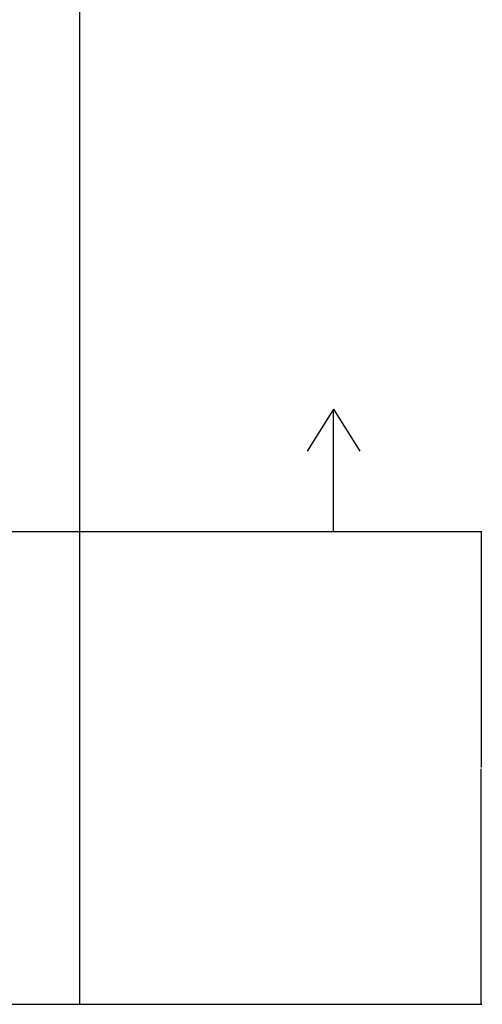
# Model space of a CAD drawing. Units: inches. Extents: x -43 to 1296, y -568 to 542.
# Tile 11 of 14: x 1187 to 1296, y -484 to -253. Entities that reach past the tile are written whole.
import ezdxf

# ---------------------------------------------------------------- set-up
doc = ezdxf.new("R2010")
doc.units = ezdxf.units.IN
doc.header["$MEASUREMENT"] = 0
doc.layers.add('A-ANNO-DIMS', color=2, linetype='Continuous', lineweight=18)
doc.layers.add('A-ANNO-SYMB', color=7, linetype='Continuous', lineweight=25)
doc.styles.get("Standard").update_dxf_attribs({"font": 'arial.ttf'})
doc.dimstyles.get("Standard").update_dxf_attribs({"dimtxt": 0.18, "dimasz": 0.18, "dimexe": 0.18, "dimexo": 0.0625, "dimgap": 0.09, "dimtad": 0, "dimtih": 1, "dimtoh": 1, "dimdec": 0, "dimzin": 0, "dimdsep": 46, "dimlunit": 3, "dimtxsty": 'Standard', "dimcen": 0.09, "dimadec": 0, "dimazin": 0, "dimtfac": 1, "dimtdec": 0, "dimtofl": 0, "dimtmove": 0, "dimatfit": 3, "dimfxl": 1, "dimtolj": 1, "dimtzin": 0, "dimarcsym": 0})

# ---------------------------------------------------------------- blocks, each defined once
blk = doc.blocks.new('*D4')
at = {"layer": 'A-ANNO-DIMS', "color": 0, "lineweight": -2, "transparency": 16777216}
for p, q in [((1184.19, -3.76), (1201.25, -3.76)), ((1201.07, -3.94), (1201.07, -240.61)), ((1201.07, -483.58), (1201.07, -246.91)), ((1184.19, -483.76), (1201.25, -483.76))]:
    blk.add_line(p, q, dxfattribs=at)
at = {"layer": 'A-ANNO-DIMS', "color": 0, "transparency": 16777216}
for points in [[(1201.04, -3.94), (1201.1, -3.94), (1201.07, -3.76)], [(1201.04, -483.58), (1201.1, -483.58), (1201.07, -483.76)]]:
    blk.add_solid(points, dxfattribs=at)
at = {"layer": 'Defpoints', "color": 0, "transparency": 16777216}
for p in [(1184.13, -3.76), (1184.13, -483.76), (1201.07, -483.76)]:
    blk.add_point(p, dxfattribs=at)
at = {"layer": 'A-ANNO-DIMS', "color": 0, "transparency": 16777216, "insert": (1201.07, -243.76), "char_height": 6, "attachment_point": 5}
blk.add_mtext("\\A1;40'", dxfattribs=at)
blk = doc.blocks.new('*D79')
at = {"layer": 'A-ANNO-DIMS', "color": 0, "lineweight": -2, "transparency": 16777216}
for p, q in [((1260.71, -372.83), (1295.51, -372.83)), ((1295.33, -373.01), (1295.33, -428.11)), ((1295.33, -483.58), (1295.33, -428.48)), ((1184.19, -483.76), (1295.51, -483.76))]:
    blk.add_line(p, q, dxfattribs=at)
at = {"layer": 'A-ANNO-DIMS', "color": 0, "transparency": 16777216}
for points in [[(1295.3, -373.01), (1295.36, -373.01), (1295.33, -372.83)], [(1295.3, -483.58), (1295.36, -483.58), (1295.33, -483.76)]]:
    blk.add_solid(points, dxfattribs=at)
at = {"layer": 'Defpoints', "color": 0, "transparency": 16777216}
for p in [(1260.65, -372.83), (1295.33, -372.83), (1184.13, -483.76)]:
    blk.add_point(p, dxfattribs=at)
at = {"layer": 'A-ANNO-DIMS', "color": 0, "transparency": 16777216, "insert": (1295.33, -428.3), "char_height": 0.18, "attachment_point": 5}
blk.add_mtext('\\A1;9\'-3"', dxfattribs=at)

msp = doc.modelspace()

# ---------------------------------------------------------------- linework, layer by layer
at = {"layer": 'A-ANNO-SYMB'}
for p, q in [((1260.65, -344.12), (1254.48, -353.96)), ((1260.65, -372.83), (1260.65, -344.12)), ((1260.65, -344.12), (1266.83, -353.96)), ((795.05, -372.83), (1260.65, -372.83))]:
    msp.add_line(p, q, dxfattribs=at)

# ---------------------------------------------------------------- dimensions: what is measured, and where the dimension line sits
at = {"layer": 'A-ANNO-DIMS'}
for base, p1, p2, override, picture, middle in [((1201.07, -483.76), (1184.13, -3.76), (1184.13, -483.76), {"dimtxt": 6, "dimclrd": 0, "dimclre": 0, "dimclrt": 0}, '*D4', (1201.07, -243.76)), ((1295.33, -372.83), (1184.13, -483.76), (1260.65, -372.83), {"dimdec": 1, "dimlfac": 1, "dimrnd": 0, "dimzin": 1, "dimdsep": 46, "dimlunit": 4, "dimfrac": 2}, '*D79', (1295.33, -428.3))]:
    dim = msp.add_linear_dim(base=base, p1=p1, p2=p2, angle=90, dimstyle='Standard', override=override, dxfattribs=at)
    dim.commit()
    dim.dimension.update_dxf_attribs({"geometry": picture, "text_midpoint": middle})

doc.saveas('drawing.dxf')
